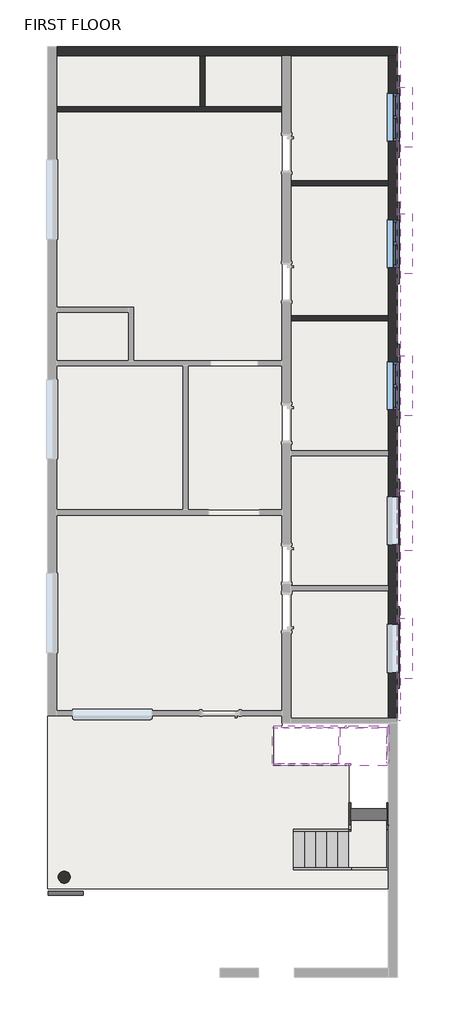
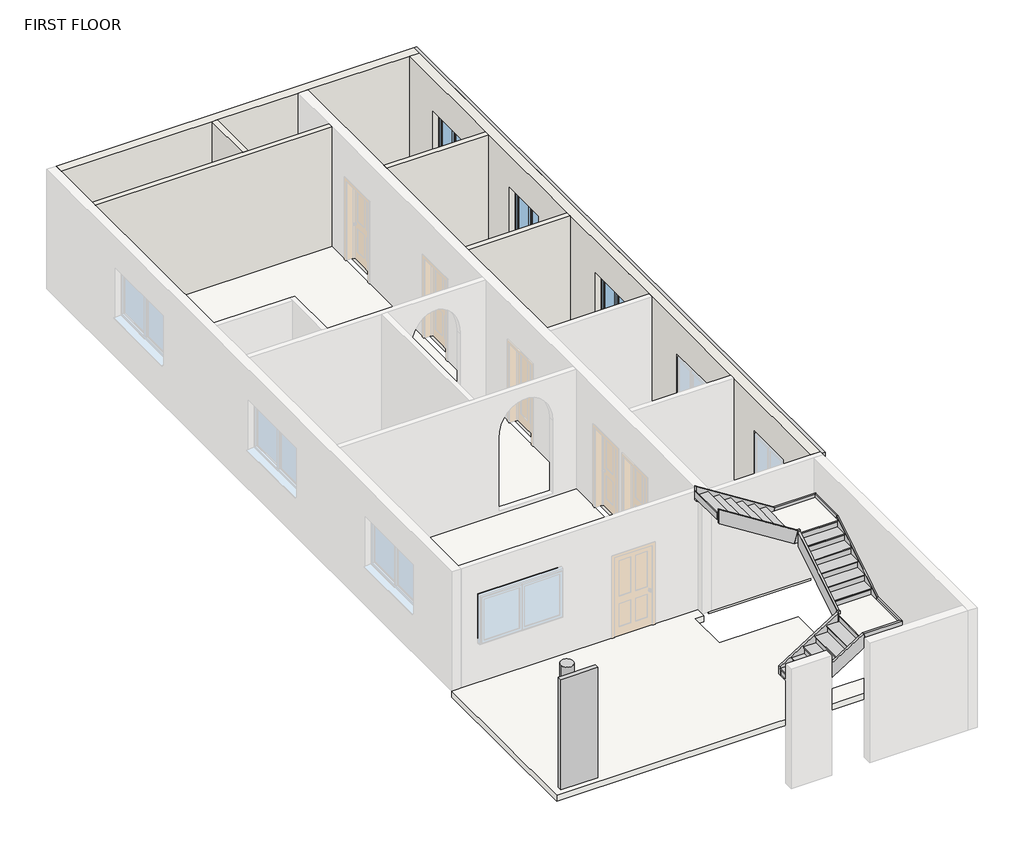
# One storey, part 2 of 2: 12 members, 8 proxies, 6 walls, 4 slabs, 3 stair flights, 3 windows, 1 column.
"""IFC4 building model written with IfcOpenShell, lengths in millimetres."""

from ifc_helpers import new_model, si_unit, frame, origin, place, context, project, spatial, polyline, outline, extrude, faceted_brep, transform, mapped, element, save
from components import generic_models_10_generic_models_10_d49a56e1, generic_models_14_generic_models_14_88c4d60d, generic_models_4_generic_models_4_2a86e6bb, generic_models_9_generic_models_9_b0d80d45, round_column_column_1_x_1_eb224a9a, non_monolithic_landing_ab58be02, non_monolithic_landing_4baf8b2c, stair_flight_8de20f2d, stair_flight_d68d3b3e, stair_flight_1ea1789e, w2_0001_windows_4_x4_9dec5fc7

model = new_model("IFC4")

# Units and contexts
model_context = context("Model", 3, world=origin())
ifc_project = project(units=[si_unit("LENGTHUNIT", "METRE", prefix="MILLI")], contexts=[model_context])

# Site, building, storey
site = spatial("IfcSite", under=ifc_project)
building = spatial("IfcBuilding", under=site)
storey = spatial("IfcBuildingStorey", under=building, Name="FIRST FLOOR", Elevation=3352.8)

# Proxies
placement = place(None, origin())
generic_models_10_generic_models_10_shape = generic_models_10_generic_models_10_d49a56e1(model_context)
element("IfcBuildingElementProxy", 1, Name="Generic Models 10 : Generic Models 10", ObjectType="Generic Models 10 : Generic Models 10", at=placement, inside=storey, context=model_context, shape_type="MappedRepresentation", body=[
    mapped(generic_models_10_generic_models_10_shape, transform((0.0, 0.0, 0.0), x_axis=(1.0, 0.0, 0.0), y_axis=(0.0, 1.0, 0.0), z_axis=(0.0, 0.0, 1.0))),
])
generic_models_14_generic_models_14_shape = generic_models_14_generic_models_14_88c4d60d(model_context)
element("IfcBuildingElementProxy", 2, Name="Generic Models 14 : Generic Models 14", ObjectType="Generic Models 14 : Generic Models 14", at=placement, inside=storey, context=model_context, shape_type="MappedRepresentation", body=[
    mapped(generic_models_14_generic_models_14_shape, transform((0.0, 0.0, 0.0), x_axis=(1.0, 0.0, 0.0), y_axis=(0.0, 1.0, 0.0), z_axis=(0.0, 0.0, 1.0))),
])
generic_models_4_generic_models_4_shape = generic_models_4_generic_models_4_2a86e6bb(model_context)
element("IfcBuildingElementProxy", 3, Name="Generic Models 4 : Generic Models 4", ObjectType="Generic Models 4 : Generic Models 4", at=placement, inside=storey, context=model_context, shape_type="MappedRepresentation", body=[
    mapped(generic_models_4_generic_models_4_shape, transform((0.0, 0.0, 0.0), x_axis=(1.0, 0.0, 0.0), y_axis=(0.0, 1.0, 0.0), z_axis=(0.0, 0.0, 1.0))),
])
element("IfcBuildingElementProxy", 4, Name="Generic Models 5 : Generic Models 4", ObjectType="Generic Models 5 : Generic Models 4", at=placement, inside=storey, context=model_context, shape_type="MappedRepresentation", body=[
    mapped(generic_models_4_generic_models_4_shape, transform((0.0, 3232.15, 0.0), x_axis=(1.0, 0.0, 0.0), y_axis=(0.0, 1.0, 0.0), z_axis=(0.0, 0.0, 1.0))),
])
element("IfcBuildingElementProxy", 5, Name="Generic Models 6 : Generic Models 4", ObjectType="Generic Models 6 : Generic Models 4", at=placement, inside=storey, context=model_context, shape_type="MappedRepresentation", body=[
    mapped(generic_models_4_generic_models_4_shape, transform((0.0, 6648.45, 0.0), x_axis=(1.0, 0.0, 0.0), y_axis=(0.0, 1.0, 0.0), z_axis=(0.0, 0.0, 1.0))),
])
element("IfcBuildingElementProxy", 6, Name="Generic Models 7 : Generic Models 4", ObjectType="Generic Models 7 : Generic Models 4", at=placement, inside=storey, context=model_context, shape_type="MappedRepresentation", body=[
    mapped(generic_models_4_generic_models_4_shape, transform((0.0, 10248.9, 0.0), x_axis=(1.0, 0.0, 0.0), y_axis=(0.0, 1.0, 0.0), z_axis=(0.0, 0.0, 1.0))),
])
element("IfcBuildingElementProxy", 7, Name="Generic Models 8 : Generic Models 4", ObjectType="Generic Models 8 : Generic Models 4", at=placement, inside=storey, context=model_context, shape_type="MappedRepresentation", body=[
    mapped(generic_models_4_generic_models_4_shape, transform((0.0, 13449.3, 0.0), x_axis=(1.0, 0.0, 0.0), y_axis=(0.0, 1.0, 0.0), z_axis=(0.0, 0.0, 1.0))),
])
generic_models_9_generic_models_9_shape = generic_models_9_generic_models_9_b0d80d45(model_context)
element("IfcBuildingElementProxy", 8, Name="Generic Models 9 : Generic Models 9", ObjectType="Generic Models 9 : Generic Models 9", at=placement, inside=storey, context=model_context, shape_type="MappedRepresentation", body=[
    mapped(generic_models_9_generic_models_9_shape, transform((0.0, 0.0, 0.0), x_axis=(1.0, 0.0, 0.0), y_axis=(0.0, 1.0, 0.0), z_axis=(0.0, 0.0, 1.0))),
])

# Column
round_column_column_1_x_1_shape = round_column_column_1_x_1_eb224a9a(model_context)
element("IfcColumn", 9, ObjectType="Round Column : COLUMN 1' X 1'", at=placement, inside=storey, context=model_context, shape_type="MappedRepresentation", body=[
    mapped(round_column_column_1_x_1_shape, transform((1692.4423568, -10961.9073314, 0.0), x_axis=(1.0, 0.0, 0.0), y_axis=(0.0, 1.0, 0.0), z_axis=(0.0, 0.0, 1.0))),
])

# Members
element("IfcMember", 10, ObjectType="Stringer - 2\" Width", at=placement, inside=storey, context=model_context, shape_type="SweptSolid", body=[
    extrude(outline(polyline([(5241.7578947, 8807.4975826), (5546.5578947, 8895.691591), (6743.6812147, 7000.2463344), (6383.1797357, 7000.2463344), (5241.7578947, 8807.4975826)])), frame((0.0, -8140.7746824, 0.0), z_axis=(0.0, 1.0, 0.0), x_axis=(0.0, 0.0, 1.0)), (0.0, 0.0, 1.0), 50.8),
])
element("IfcMember", 11, ObjectType="Stringer - 2\" Width", at=placement, inside=storey, context=model_context, shape_type="SweptSolid", body=[
    extrude(outline(polyline([(5241.7578947, 8807.4975826), (5546.5578947, 8895.691591), (6743.6812147, 7000.2463344), (6383.1797357, 7000.2463344), (5241.7578947, 8807.4975826)])), frame((0.0, -7175.5746824, 0.0), z_axis=(0.0, 1.0, 0.0), x_axis=(0.0, 0.0, 1.0)), (0.0, 0.0, 1.0), 50.8),
])
element("IfcMember", 12, ObjectType="Stringer - 2\" Width", at=placement, inside=storey, context=model_context, shape_type="SweptSolid", body=[
    extrude(outline(polyline([(-9668.6259307, 4182.9789474), (-9756.819939, 4487.7789474), (-8140.7746824, 5508.4391095), (-8140.7746824, 5147.9376305), (-9668.6259307, 4182.9789474)])), frame((8906.0423568, 0.0, 0.0), z_axis=(1.0, 0.0, 0.0), x_axis=(0.0, 1.0, 0.0)), (0.0, 0.0, 1.0), 50.8),
])
element("IfcMember", 13, ObjectType="Stringer - 2\" Width", at=placement, inside=storey, context=model_context, shape_type="SweptSolid", body=[
    extrude(outline(polyline([(-9668.6259307, 4182.9789474), (-9756.819939, 4487.7789474), (-8080.419939, 5546.5578947), (-7992.2259307, 5241.7578947), (-9668.6259307, 4182.9789474)])), frame((9871.2423568, 0.0, 0.0), z_axis=(1.0, 0.0, 0.0), x_axis=(0.0, 1.0, 0.0)), (0.0, 0.0, 1.0), 50.8),
])
element("IfcMember", 14, ObjectType="Stringer - 2\" Width", at=placement, inside=storey, context=model_context, shape_type="SweptSolid", body=[
    extrude(outline(polyline([(5546.5578947, 8895.691591), (5241.7578947, 8807.4975826), (5241.7578947, 8956.8423568), (5546.5578947, 8956.8423568), (5546.5578947, 8895.691591)])), frame((0.0, -8140.7746824, 0.0), z_axis=(0.0, 1.0, 0.0), x_axis=(0.0, 0.0, 1.0)), (0.0, 0.0, 1.0), 50.8),
])
element("IfcMember", 15, ObjectType="Stringer - 2\" Width", at=placement, inside=storey, context=model_context, shape_type="Brep", body=[
    faceted_brep([(9871.2423568, -8080.419939, 5546.5578947), (9922.0423568, -8080.419939, 5546.5578947), (9922.0423568, -7124.7746824, 5546.5578947), (9871.2423568, -7175.5746824, 5546.5578947), (9871.2423568, -7992.2259307, 5241.7578947), (9871.2423568, -7175.5746824, 5241.7578947), (9922.0423568, -7992.2259307, 5241.7578947), (9922.0423568, -7124.7746824, 5241.7578947)], [[[0, 1, 2, 3]], [[4, 0, 3, 5]], [[6, 4, 5, 7]], [[1, 6, 7, 2]], [[1, 0, 4, 6]], [[2, 7, 5, 3]]]),
])
element("IfcMember", 16, ObjectType="Stringer - 2\" Width", at=placement, inside=storey, context=model_context, shape_type="Brep", body=[
    faceted_brep([(9871.2423568, -7175.5746824, 5546.5578947), (9922.0423568, -7124.7746824, 5546.5578947), (8895.691591, -7124.7746824, 5546.5578947), (8895.691591, -7175.5746824, 5546.5578947), (9871.2423568, -7175.5746824, 5241.7578947), (8807.4975826, -7175.5746824, 5241.7578947), (9922.0423568, -7124.7746824, 5241.7578947), (8807.4975826, -7124.7746824, 5241.7578947)], [[[0, 1, 2, 3]], [[4, 0, 3, 5]], [[6, 4, 5, 7]], [[1, 6, 7, 2]], [[1, 0, 4, 6]], [[2, 7, 5, 3]]]),
])
element("IfcMember", 17, ObjectType="Stringer - 2\" Width", at=placement, inside=storey, context=model_context, shape_type="SweptSolid", body=[
    extrude(outline(polyline([(3567.3443726, 7509.0423568), (3352.8, 7509.0423568), (3352.8, 7740.1411085), (4089.1586831, 8906.0423568), (4449.6601621, 8906.0423568), (3567.3443726, 7509.0423568)])), frame((0.0, -9806.2073314, 0.0), z_axis=(0.0, 1.0, 0.0), x_axis=(0.0, 0.0, 1.0)), (0.0, 0.0, 1.0), 50.8),
])
element("IfcMember", 18, ObjectType="Stringer - 2\" Width", at=placement, inside=storey, context=model_context, shape_type="SweptSolid", body=[
    extrude(outline(polyline([(3567.3443726, 7509.0423568), (3352.8, 7509.0423568), (3352.8, 7740.1411085), (4182.9789474, 9054.5911085), (4487.7789474, 8966.3971001), (3567.3443726, 7509.0423568)])), frame((0.0, -10771.4073314, 0.0), z_axis=(0.0, 1.0, 0.0), x_axis=(0.0, 0.0, 1.0)), (0.0, 0.0, 1.0), 50.8),
])
element("IfcMember", 19, ObjectType="Stringer - 2\" Width", at=placement, inside=storey, context=model_context, shape_type="SweptSolid", body=[
    extrude(outline(polyline([(-9756.819939, 4487.7789474), (-9668.6259307, 4182.9789474), (-9806.2073314, 4182.9789474), (-9806.2073314, 4487.7789474), (-9756.819939, 4487.7789474)])), frame((8906.0423568, 0.0, 0.0), z_axis=(1.0, 0.0, 0.0), x_axis=(0.0, 1.0, 0.0)), (0.0, 0.0, 1.0), 50.8),
])
element("IfcMember", 20, ObjectType="Stringer - 2\" Width", at=placement, inside=storey, context=model_context, shape_type="Brep", body=[
    faceted_brep([(8966.3971001, -10720.6073314, 4487.7789474), (8966.3971001, -10771.4073314, 4487.7789474), (9922.0423568, -10771.4073314, 4487.7789474), (9871.2423568, -10720.6073314, 4487.7789474), (9054.5911085, -10720.6073314, 4182.9789474), (9871.2423568, -10720.6073314, 4182.9789474), (9054.5911085, -10771.4073314, 4182.9789474), (9922.0423568, -10771.4073314, 4182.9789474)], [[[0, 1, 2, 3]], [[4, 0, 3, 5]], [[6, 4, 5, 7]], [[1, 6, 7, 2]], [[1, 0, 4, 6]], [[2, 7, 5, 3]]]),
])
element("IfcMember", 21, ObjectType="Stringer - 2\" Width", at=placement, inside=storey, context=model_context, shape_type="Brep", body=[
    faceted_brep([(9871.2423568, -10720.6073314, 4487.7789474), (9922.0423568, -10771.4073314, 4487.7789474), (9922.0423568, -9756.819939, 4487.7789474), (9871.2423568, -9756.819939, 4487.7789474), (9871.2423568, -10720.6073314, 4182.9789474), (9871.2423568, -9668.6259307, 4182.9789474), (9922.0423568, -10771.4073314, 4182.9789474), (9922.0423568, -9668.6259307, 4182.9789474)], [[[0, 1, 2, 3]], [[4, 0, 3, 5]], [[6, 4, 5, 7]], [[1, 6, 7, 2]], [[1, 0, 4, 6]], [[2, 7, 5, 3]]]),
])

# Slabs
element("IfcSlab", 22, ObjectType="FLOORING 6\"", at=placement, inside=storey, context=model_context, shape_type="SweptSolid", body=[
    extrude(outline(polyline([(5134.1423568, 9840.6926686), (5134.1423568, 8545.2926686), (1501.9423568, 8545.2926686), (1501.9423568, 9840.6926686), (5134.1423568, 9840.6926686)])), frame((0.0, 0.0, 3200.4), z_axis=(0.0, 0.0, 1.0), x_axis=(1.0, 0.0, 0.0)), (0.0, 0.0, 1.0), 152.4),
    extrude(outline(polyline([(7216.9423568, 9840.6926686), (7216.9423568, 8545.2926686), (5261.1423568, 8545.2926686), (5261.1423568, 9840.6926686), (7216.9423568, 9840.6926686)])), frame((0.0, 0.0, 3200.4), z_axis=(0.0, 0.0, 1.0), x_axis=(1.0, 0.0, 0.0)), (0.0, 0.0, 1.0), 152.4),
    extrude(outline(polyline([(9909.3423568, 9840.6926686), (9909.3423568, 6665.6926686), (7445.5423568, 6665.6926686), (7445.5423568, 9840.6926686), (9909.3423568, 9840.6926686)])), frame((0.0, 0.0, 3200.4), z_axis=(0.0, 0.0, 1.0), x_axis=(1.0, 0.0, 0.0)), (0.0, 0.0, 1.0), 152.4),
    extrude(outline(polyline([(9909.3423568, 6538.6926686), (9909.3423568, 3249.3926686), (7445.5423568, 3249.3926686), (7445.5423568, 6538.6926686), (9909.3423568, 6538.6926686)])), frame((0.0, 0.0, 3200.4), z_axis=(0.0, 0.0, 1.0), x_axis=(1.0, 0.0, 0.0)), (0.0, 0.0, 1.0), 152.4),
    extrude(outline(polyline([(9909.3423568, 3122.3926686), (9909.3423568, -166.9073314), (7445.5423568, -166.9073314), (7445.5423568, 3122.3926686), (9909.3423568, 3122.3926686)])), frame((0.0, 0.0, 3200.4), z_axis=(0.0, 0.0, 1.0), x_axis=(1.0, 0.0, 0.0)), (0.0, 0.0, 1.0), 152.4),
    extrude(outline(polyline([(9909.3423568, -293.9073314), (9909.3423568, -3583.2073314), (7445.5423568, -3583.2073314), (7445.5423568, -293.9073314), (9909.3423568, -293.9073314)])), frame((0.0, 0.0, 3200.4), z_axis=(0.0, 0.0, 1.0), x_axis=(1.0, 0.0, 0.0)), (0.0, 0.0, 1.0), 152.4),
    extrude(outline(polyline([(9909.3423568, -3710.2073314), (9909.3423568, -6936.0073314), (7445.5423568, -6936.0073314), (7445.5423568, -3710.2073314), (9909.3423568, -3710.2073314)])), frame((0.0, 0.0, 3200.4), z_axis=(0.0, 0.0, 1.0), x_axis=(1.0, 0.0, 0.0)), (0.0, 0.0, 1.0), 152.4),
    extrude(outline(polyline([(7216.9423568, -1792.5073314), (7216.9423568, -6745.5073314), (1501.9423568, -6745.5073314), (1501.9423568, -1792.5073314), (7216.9423568, -1792.5073314)])), frame((0.0, 0.0, 3200.4), z_axis=(0.0, 0.0, 1.0), x_axis=(1.0, 0.0, 0.0)), (0.0, 0.0, 1.0), 152.4),
    extrude(outline(polyline([(4702.3423568, 1992.0926686), (4702.3423568, -1665.5073314), (1501.9423568, -1665.5073314), (1501.9423568, 1992.0926686), (4702.3423568, 1992.0926686)])), frame((0.0, 0.0, 3200.4), z_axis=(0.0, 0.0, 1.0), x_axis=(1.0, 0.0, 0.0)), (0.0, 0.0, 1.0), 152.4),
    extrude(outline(polyline([(7216.9423568, 1992.0926686), (7216.9423568, -1665.5073314), (4829.3423568, -1665.5073314), (4829.3423568, 1992.0926686), (7216.9423568, 1992.0926686)])), frame((0.0, 0.0, 3200.4), z_axis=(0.0, 0.0, 1.0), x_axis=(1.0, 0.0, 0.0)), (0.0, 0.0, 1.0), 152.4),
    extrude(outline(polyline([(3330.7423568, 3338.2926686), (3330.7423568, 2119.0926686), (1501.9423568, 2119.0926686), (1501.9423568, 3338.2926686), (3330.7423568, 3338.2926686)])), frame((0.0, 0.0, 3200.4), z_axis=(0.0, 0.0, 1.0), x_axis=(1.0, 0.0, 0.0)), (0.0, 0.0, 1.0), 152.4),
    extrude(outline(polyline([(7216.9423568, 8418.2926686), (7216.9423568, 2119.0926686), (3457.7423568, 2119.0926686), (3457.7423568, 3465.2926686), (1501.9423568, 3465.2926686), (1501.9423568, 8418.2926686), (7216.9423568, 8418.2926686)])), frame((0.0, 0.0, 3200.4), z_axis=(0.0, 0.0, 1.0), x_axis=(1.0, 0.0, 0.0)), (0.0, 0.0, 1.0), 152.4),
])
element("IfcSlab", 23, ObjectType="FLOORING 6\"", at=placement, inside=storey, context=model_context, shape_type="SweptSolid", body=[
    extrude(outline(polyline([(7216.9423568, -6872.5073314), (7216.9423568, -7124.7746824), (7000.2463344, -7124.7746824), (7000.2463344, -8140.7746824), (8906.0423568, -8140.7746824), (8906.0423568, -9755.4073314), (7509.0423568, -9755.4073314), (7509.0423568, -10771.4073314), (9909.3423568, -10771.4073314), (9909.3423568, -11254.0073314), (1273.3423568, -11254.0073314), (1273.3423568, -6872.5073314), (1501.9423568, -6872.5073314), (7216.9423568, -6872.5073314)])), frame((0.0, 0.0, 3200.4), z_axis=(0.0, 0.0, 1.0), x_axis=(1.0, 0.0, 0.0)), (0.0, 0.0, 1.0), 152.4),
])
non_monolithic_landing_shape = non_monolithic_landing_ab58be02(model_context)
element("IfcSlab", 24, ObjectType="Non-Monolithic Landing", at=placement, inside=storey, context=model_context, shape_type="MappedRepresentation", body=[
    mapped(non_monolithic_landing_shape, transform((0.0, 0.0, 0.0), x_axis=(1.0, 0.0, 0.0), y_axis=(0.0, 1.0, 0.0), z_axis=(0.0, 0.0, 1.0))),
])
non_monolithic_landing_2_shape = non_monolithic_landing_4baf8b2c(model_context)
element("IfcSlab", 25, ObjectType="Non-Monolithic Landing", at=placement, inside=storey, context=model_context, shape_type="MappedRepresentation", body=[
    mapped(non_monolithic_landing_2_shape, transform((0.0, 0.0, 0.0), x_axis=(1.0, 0.0, 0.0), y_axis=(0.0, 1.0, 0.0), z_axis=(0.0, 0.0, 1.0))),
])

# Stair flights
stair_flight_shape = stair_flight_8de20f2d(model_context)
element("IfcStairFlight", 26, ObjectType="2\" Tread 1\" Nosing 1/4\" Riser", at=placement, inside=storey, context=model_context, shape_type="MappedRepresentation", body=[
    mapped(stair_flight_shape, transform((0.0, 0.0, 0.0), x_axis=(1.0, 0.0, 0.0), y_axis=(0.0, 1.0, 0.0), z_axis=(0.0, 0.0, 1.0))),
])
stair_flight_2_shape = stair_flight_d68d3b3e(model_context)
element("IfcStairFlight", 27, ObjectType="2\" Tread 1\" Nosing 1/4\" Riser", at=placement, inside=storey, context=model_context, shape_type="MappedRepresentation", body=[
    mapped(stair_flight_2_shape, transform((0.0, 0.0, 0.0), x_axis=(1.0, 0.0, 0.0), y_axis=(0.0, 1.0, 0.0), z_axis=(0.0, 0.0, 1.0))),
])
stair_flight_3_shape = stair_flight_1ea1789e(model_context)
element("IfcStairFlight", 28, ObjectType="2\" Tread 1\" Nosing 1/4\" Riser", at=placement, inside=storey, context=model_context, shape_type="MappedRepresentation", body=[
    mapped(stair_flight_3_shape, transform((0.0, 0.0, 0.0), x_axis=(1.0, 0.0, 0.0), y_axis=(0.0, 1.0, 0.0), z_axis=(0.0, 0.0, 1.0))),
])

# Walls
element("IfcWall", 29, ObjectType="INNER WALL 5\"", at=placement, inside=storey, context=model_context, shape_type="SweptSolid", body=[
    extrude(outline(polyline([(7445.5423568, 6665.6926686), (9909.3423568, 6665.6926686), (9909.3423568, 6538.6926686), (7445.5423568, 6538.6926686), (7445.5423568, 6665.6926686)])), frame((0.0, 0.0, 3352.8), z_axis=(0.0, 0.0, 1.0), x_axis=(1.0, 0.0, 0.0)), (0.0, 0.0, 1.0), 3048.0),
])
element("IfcWall", 30, ObjectType="INNER WALL 5\"", at=placement, inside=storey, context=model_context, shape_type="SweptSolid", body=[
    extrude(outline(polyline([(7445.5423568, 3249.3926686), (9909.3423568, 3249.3926686), (9909.3423568, 3122.3926686), (7445.5423568, 3122.3926686), (7445.5423568, 3249.3926686)])), frame((0.0, 0.0, 3352.8), z_axis=(0.0, 0.0, 1.0), x_axis=(1.0, 0.0, 0.0)), (0.0, 0.0, 1.0), 3048.0),
])
element("IfcWall", 31, ObjectType="INNER WALL 5\"", at=placement, inside=storey, context=model_context, shape_type="Brep", body=[
    faceted_brep([(7216.9423568, 8545.2926686, 3352.8), (5261.1423568, 8545.2926686, 3352.8), (5134.1423568, 8545.2926686, 3352.8), (1501.9423568, 8545.2926686, 3352.8), (1501.9423568, 8545.2926686, 6400.8), (5134.1423568, 8545.2926686, 6400.8), (5261.1423568, 8545.2926686, 6400.8), (7216.9423568, 8545.2926686, 6400.8), (7216.9423568, 8418.2926686, 3352.8), (7216.9423568, 8418.2926686, 6400.8), (1501.9423568, 8418.2926686, 6400.8), (1501.9423568, 8418.2926686, 3352.8)], [[[0, 1, 2, 3, 4, 5, 6, 7]], [[8, 9, 10, 11]], [[3, 2, 1, 0, 8, 11]], [[7, 6, 5, 4, 10, 9]], [[4, 3, 11, 10]], [[0, 7, 9, 8]]]),
])
element("IfcWall", 32, ObjectType="INNER WALL 5\"", at=placement, inside=storey, context=model_context, shape_type="SweptSolid", body=[
    extrude(outline(polyline([(5134.1423568, 8545.2926686), (5134.1423568, 9840.6926686), (5261.1423568, 9840.6926686), (5261.1423568, 8545.2926686), (5134.1423568, 8545.2926686)])), frame((0.0, 0.0, 3352.8), z_axis=(0.0, 0.0, 1.0), x_axis=(1.0, 0.0, 0.0)), (0.0, 0.0, 1.0), 3048.0),
])
element("IfcWall", 33, ObjectType="OUTER WALL 9\"", at=placement, inside=storey, context=model_context, shape_type="Brep", body=[
    faceted_brep([(1501.9423568, 9840.6926686, 3352.8), (5134.1423568, 9840.6926686, 3352.8), (5261.1423568, 9840.6926686, 3352.8), (7216.9423568, 9840.6926686, 3352.8), (7445.5423568, 9840.6926686, 3352.8), (9909.3423568, 9840.6926686, 3352.8), (10137.9423568, 9840.6926686, 3352.8), (10137.9423568, 9840.6926686, 6400.8), (9909.3423568, 9840.6926686, 6400.8), (7445.5423568, 9840.6926686, 6400.8), (7216.9423568, 9840.6926686, 6400.8), (5261.1423568, 9840.6926686, 6400.8), (5134.1423568, 9840.6926686, 6400.8), (1501.9423568, 9840.6926686, 6400.8), (1501.9423568, 10069.2926686, 3352.8), (1501.9423568, 10069.2926686, 6400.8), (10137.9423568, 10069.2926686, 6400.8), (10137.9423568, 10069.2926686, 3352.8)], [[[0, 1, 2, 3, 4, 5, 6, 7, 8, 9, 10, 11, 12, 13]], [[14, 15, 16, 17]], [[6, 5, 4, 3, 2, 1, 0, 14, 17]], [[13, 12, 11, 10, 9, 8, 7, 16, 15]], [[0, 13, 15, 14]], [[7, 6, 17, 16]]]),
])
element("IfcWall", 34, ObjectType="OUTER WALL 9\"", at=placement, inside=storey, context=model_context, shape_type="Brep", body=[
    faceted_brep([(10137.9423568, -6936.0073314, 3352.8), (10137.9423568, 9840.6926686, 3352.8), (10137.9423568, 9840.6926686, 6400.8), (10137.9423568, -6936.0073314, 6400.8), (10137.9423568, -1328.9573314, 4352.8), (10137.9423568, -2548.1573314, 4352.8), (10137.9423568, -2548.1573314, 5572.0), (10137.9423568, -1328.9573314, 5572.0), (10137.9423568, 868.1426686, 4352.8), (10137.9423568, 868.1426686, 5572.0), (10137.9423568, 2087.3426686, 5572.0), (10137.9423568, 2087.3426686, 4352.8), (10137.9423568, 4468.5926686, 4352.8), (10137.9423568, 4468.5926686, 5572.0), (10137.9423568, 5687.7926686, 5572.0), (10137.9423568, 5687.7926686, 4352.8), (10137.9423568, 7668.9926686, 4352.8), (10137.9423568, 7668.9926686, 5572.0), (10137.9423568, 8888.1926686, 5572.0), (10137.9423568, 8888.1926686, 4352.8), (10137.9423568, -4561.1073314, 4352.8), (10137.9423568, -5780.3073314, 4352.8), (10137.9423568, -5780.3073314, 5572.0), (10137.9423568, -4561.1073314, 5572.0), (9909.3423568, -6936.0073314, 3352.8), (9909.3423568, -6936.0073314, 6400.8), (9909.3423568, -3710.2073314, 6400.8), (9909.3423568, -3583.2073314, 6400.8), (9909.3423568, -293.9073314, 6400.8), (9909.3423568, -166.9073314, 6400.8), (9909.3423568, 3122.3926686, 6400.8), (9909.3423568, 3249.3926686, 6400.8), (9909.3423568, 6538.6926686, 6400.8), (9909.3423568, 6665.6926686, 6400.8), (9909.3423568, 9840.6926686, 6400.8), (9909.3423568, 9840.6926686, 3352.8), (9909.3423568, 6665.6926686, 3352.8), (9909.3423568, 6538.6926686, 3352.8), (9909.3423568, 3249.3926686, 3352.8), (9909.3423568, 3122.3926686, 3352.8), (9909.3423568, -166.9073314, 3352.8), (9909.3423568, -293.9073314, 3352.8), (9909.3423568, -3583.2073314, 3352.8), (9909.3423568, -3710.2073314, 3352.8), (9909.3423568, -1328.9573314, 4352.8), (9909.3423568, -1328.9573314, 5572.0), (9909.3423568, -2548.1573314, 5572.0), (9909.3423568, -2548.1573314, 4352.8), (9909.3423568, 868.1426686, 4352.8), (9909.3423568, 2087.3426686, 4352.8), (9909.3423568, 2087.3426686, 5572.0), (9909.3423568, 868.1426686, 5572.0), (9909.3423568, 4468.5926686, 4352.8), (9909.3423568, 5687.7926686, 4352.8), (9909.3423568, 5687.7926686, 5572.0), (9909.3423568, 4468.5926686, 5572.0), (9909.3423568, 7668.9926686, 4352.8), (9909.3423568, 8888.1926686, 4352.8), (9909.3423568, 8888.1926686, 5572.0), (9909.3423568, 7668.9926686, 5572.0), (9909.3423568, -4561.1073314, 4352.8), (9909.3423568, -4561.1073314, 5572.0), (9909.3423568, -5780.3073314, 5572.0), (9909.3423568, -5780.3073314, 4352.8)], [[[0, 1, 2, 3], [4, 5, 6, 7], [8, 9, 10, 11], [12, 13, 14, 15], [16, 17, 18, 19], [20, 21, 22, 23]], [[24, 25, 26, 27, 28, 29, 30, 31, 32, 33, 34, 35, 36, 37, 38, 39, 40, 41, 42, 43], [44, 45, 46, 47], [48, 49, 50, 51], [52, 53, 54, 55], [56, 57, 58, 59], [60, 61, 62, 63]], [[1, 0, 24, 43, 42, 41, 40, 39, 38, 37, 36, 35]], [[3, 2, 34, 33, 32, 31, 30, 29, 28, 27, 26, 25]], [[2, 1, 35, 34]], [[0, 3, 25, 24]], [[45, 44, 4, 7]], [[46, 45, 7, 6]], [[47, 46, 6, 5]], [[44, 47, 5, 4]], [[9, 8, 48, 51]], [[10, 9, 51, 50]], [[11, 10, 50, 49]], [[8, 11, 49, 48]], [[13, 12, 52, 55]], [[14, 13, 55, 54]], [[15, 14, 54, 53]], [[12, 15, 53, 52]], [[17, 16, 56, 59]], [[18, 17, 59, 58]], [[19, 18, 58, 57]], [[16, 19, 57, 56]], [[61, 60, 20, 23]], [[62, 61, 23, 22]], [[63, 62, 22, 21]], [[60, 63, 21, 20]]]),
])

# Windows
w2_0001_windows_4_x4_shape = w2_0001_windows_4_x4_9dec5fc7(model_context)
element("IfcWindow", 35, ObjectType="w2.0001 : WINDOWS 4' X4'", at=placement, inside=storey, context=model_context, shape_type="MappedRepresentation", body=[
    mapped(w2_0001_windows_4_x4_shape, transform((10023.6423568, 1477.7426686, 3352.8), x_axis=(0.0, 1.0, 0.0), y_axis=(-1.0, 0.0, 0.0), z_axis=(0.0, 0.0, 1.0))),
])
element("IfcWindow", 36, ObjectType="w2.0001 : WINDOWS 4' X4'", at=placement, inside=storey, context=model_context, shape_type="MappedRepresentation", body=[
    mapped(w2_0001_windows_4_x4_shape, transform((10023.6423568, 5078.1926686, 3352.8), x_axis=(0.0, 1.0, 0.0), y_axis=(-1.0, 0.0, 0.0), z_axis=(0.0, 0.0, 1.0))),
])
element("IfcWindow", 37, ObjectType="w2.0001 : WINDOWS 4' X4'", at=placement, inside=storey, context=model_context, shape_type="MappedRepresentation", body=[
    mapped(w2_0001_windows_4_x4_shape, transform((10023.6423568, 8278.5926686, 3352.8), x_axis=(0.0, 1.0, 0.0), y_axis=(-1.0, 0.0, 0.0), z_axis=(0.0, 0.0, 1.0))),
])

save(model, "model.ifc")

# Revit data of these elements
# Type "Round Column : COLUMN 1' X 1'"
#   Assembly Code = "B1010200"
#   Diameter = 1' - 0"
#   Offset Base = 0' - 0"
#   Offset Top = 0' - 0"
#   Material = CREAM BEIGE COLOUR
# Type "FLOORING 6\""
#   Assembly Code = "B1010"
#   Function = 0
#   Layers, outside or top first: 0' - 6" "CARPET MATERIAL FLOORING" (function 1)
# Type "INNER WALL 5\""
#   Assembly Code = "B2010"
#   Layers, outside or top first: 0' - 5" "CREAM BEIGE COLOUR" (function 1)
# Type "OUTER WALL 9\""
#   Assembly Code = "B2010"
#   Layers, outside or top first: 0' - 9" "CREAM BEIGE COLOUR" (function 1)
# Type "w2.0001 : WINDOWS 4' X4'"
#   Type Mark = "22"
#   Operation = "DoublePanelVertical"
#   Keynote = "16.05.01"
#   Analytic Construction = "<None>"
#   Rough Width = 4' - 0"
#   Rough Height = 4' - 0"
#   Rahmentiefe = 0' - 2.3622"
#   Rahmenhöhe unten = 0' - 3.14961"
#   Rahmehöhe oben = 0' - 3.14961"
#   Rahmenbreite = 0' - 2.3622"
#   Height = 4' - 0"
#   Flügeltiefe = 0' - 2.3622"
#   Flügelbreite = 0' - 2.3622"
#   Einbautiefe (von außen) [instance default] = 0' - 5.51181"
#   Width = 4' - 0"
#   Kippflügel [instance default] = yes
#   Drehflügel im Grundriß darstellen [instance default] = no
#   Drehflügel [instance default] = yes
#   Define Thermal Properties by = 1
#   Rahmen [instance default] = none
#   Glas [instance default] = none
#   Flügel [instance default] = none
#   Fensterbank aussen [instance default] = none
#   Fensterbank innen [instance default] = none
#   Wall Closure = (empty or 0)
# Element 1 (IfcBuildingElementProxy, "Generic Models 10 : Generic Models 10")
#   Phase Created = New Construction
#   Materials on its faces: "Clad - White"
# Element 2 (IfcBuildingElementProxy, "Generic Models 14 : Generic Models 14")
#   Phase Created = New Construction
# Element 3 (IfcBuildingElementProxy, "Generic Models 4 : Generic Models 4")
#   Phase Created = New Construction
#   Materials on its faces: "Clad - White"
# Element 4 (IfcBuildingElementProxy, "Generic Models 5 : Generic Models 4")
#   Phase Created = New Construction
#   Materials on its faces: "Clad - White"
# Element 5 (IfcBuildingElementProxy, "Generic Models 6 : Generic Models 4")
#   Phase Created = New Construction
#   Materials on its faces: "Clad - White"
# Element 6 (IfcBuildingElementProxy, "Generic Models 7 : Generic Models 4")
#   Phase Created = New Construction
#   Materials on its faces: "Clad - White"
# Element 7 (IfcBuildingElementProxy, "Generic Models 8 : Generic Models 4")
#   Phase Created = New Construction
#   Materials on its faces: "Clad - White"
# Element 8 (IfcBuildingElementProxy, "Generic Models 9 : Generic Models 9")
#   Phase Created = New Construction
#   Materials on its faces: "WOOD MATERIAL 9\""
# Element 9 (IfcColumn, "Round Column : COLUMN 1' X 1'")
#   Phase Created = New Construction
#   Materials on its faces: "CREAM BEIGE COLOUR"
# Elements 10, 12, 17, 18, 19, 20 (IfcMember, "Stringer - 2\" Width")
#   Phase Created = New Construction
#   Materials on its faces: "MARBLE STAIRS 6\""
# Elements 11, 13, 14, 15, 16, 21 (IfcMember, "Stringer - 2\" Width")
#   Phase Created = New Construction
# Elements 22, 23 (IfcSlab, "FLOORING 6\"")
#   Height Offset From Level = 0' - 0"
#   Phase Created = New Construction
#   Materials on its faces: "CARPET MATERIAL FLOORING"
# Elements 24, 25 (IfcSlab, "Non-Monolithic Landing")
#   Phase Created = New Construction
#   Materials on its faces: "MARBLE STAIRS 6\""
# Elements 26, 27, 28 (IfcStairFlight, "2\" Tread 1\" Nosing 1/4\" Riser")
#   Phase Created = New Construction
#   Materials on its faces: "MARBLE STAIRS 6\""
# Element 29 (IfcWall, "INNER WALL 5\"")
#   Top Offset = 0' - 0"
#   Base Offset = 0' - 0"
#   Unconnected Height = 10' - 0"
#   wall height = 10' - 0"
#   Phase Created = New Construction
#   Base Constraint = FIRST FLOOR
#   Materials on its faces: "CREAM BEIGE COLOUR"
# Elements 30, 31, 32 (IfcWall, "INNER WALL 5\"")
#   Top Offset = 0' - 0"
#   Base Offset = 0' - 0"
#   wall height = 10' - 0"
#   Phase Created = New Construction
#   Base Constraint = FIRST FLOOR
#   Top Constraint = Level 4
#   Materials on its faces: "CREAM BEIGE COLOUR"
# Element 33 (IfcWall, "OUTER WALL 9\"")
#   Top Offset = 0' - 0"
#   Base Offset = 0' - 0"
#   Unconnected Height = 10' - 0"
#   wall height = 10' - 0"
#   Phase Created = New Construction
#   Base Constraint = FIRST FLOOR
#   Materials on its faces: "CREAM BEIGE COLOUR"
# Element 34 (IfcWall, "OUTER WALL 9\"")
#   Top Offset = 0' - 0"
#   Base Offset = 0' - 0"
#   wall height = 10' - 0"
#   Phase Created = New Construction
#   Base Constraint = FIRST FLOOR
#   Top Constraint = Level 4
#   Materials on its faces: "CREAM BEIGE COLOUR"
# Element 35 (IfcWindow, "w2.0001 : WINDOWS 4' X4'")
#   Mark = "10"
#   Einbautiefe (von außen) = 0' - 5.51181"
#   Kippflügel = yes
#   Drehflügel im Grundriß darstellen = no
#   Drehflügel = yes
#   Rahmen = none
#   Glas = none
#   Flügel = none
#   Fensterbank innen = none
#   Fensterbank aussen = none
#   Phase Created = New Construction
#   Materials on its faces: "Fenster - Kunststoff", "Fenster - Kunststoff weiss", "Glass", "Fenster - Holz"
# Element 36 (IfcWindow, "w2.0001 : WINDOWS 4' X4'")
#   Mark = "11"
#   Einbautiefe (von außen) = 0' - 5.51181"
#   Kippflügel = yes
#   Drehflügel im Grundriß darstellen = no
#   Drehflügel = yes
#   Rahmen = none
#   Glas = none
#   Flügel = none
#   Fensterbank innen = none
#   Fensterbank aussen = none
#   Phase Created = New Construction
#   Materials on its faces: "Fenster - Kunststoff", "Fenster - Kunststoff weiss", "Glass", "Fenster - Holz"
# Element 37 (IfcWindow, "w2.0001 : WINDOWS 4' X4'")
#   Mark = "12"
#   Einbautiefe (von außen) = 0' - 5.51181"
#   Kippflügel = yes
#   Drehflügel im Grundriß darstellen = no
#   Drehflügel = yes
#   Rahmen = none
#   Glas = none
#   Flügel = none
#   Fensterbank innen = none
#   Fensterbank aussen = none
#   Phase Created = New Construction
#   Materials on its faces: "Fenster - Kunststoff", "Fenster - Kunststoff weiss", "Glass", "Fenster - Holz"
# Materials
#   "CREAM BEIGE COLOUR": class "Generic", colour RGB 120 120 120, transparency 0, Cost = 0
#   "CARPET MATERIAL FLOORING": class "Generic", colour RGB 120 120 120, transparency 0, Cost = 0
#   "Clad - White": class "Wood", colour RGB 242 242 238, transparency 0, Cost = 0
#   "WOOD MATERIAL 9\"": class "Generic", colour RGB 120 120 120, transparency 0, Cost = 0
#   "MARBLE STAIRS 6\"": class "Generic", colour RGB 120 120 120, transparency 0, Cost = 0
#   "Fenster - Kunststoff": colour RGB 249 249 249, transparency 0
#   "Fenster - Kunststoff weiss": colour RGB 249 249 249, transparency 0
#   "Glass": class "Glass", colour RGB 0 128 192, transparency 0.75, Description = "Soda Lime Glass", Cost = 0
#   "Fenster - Holz": colour RGB 216 135 75, transparency 0
